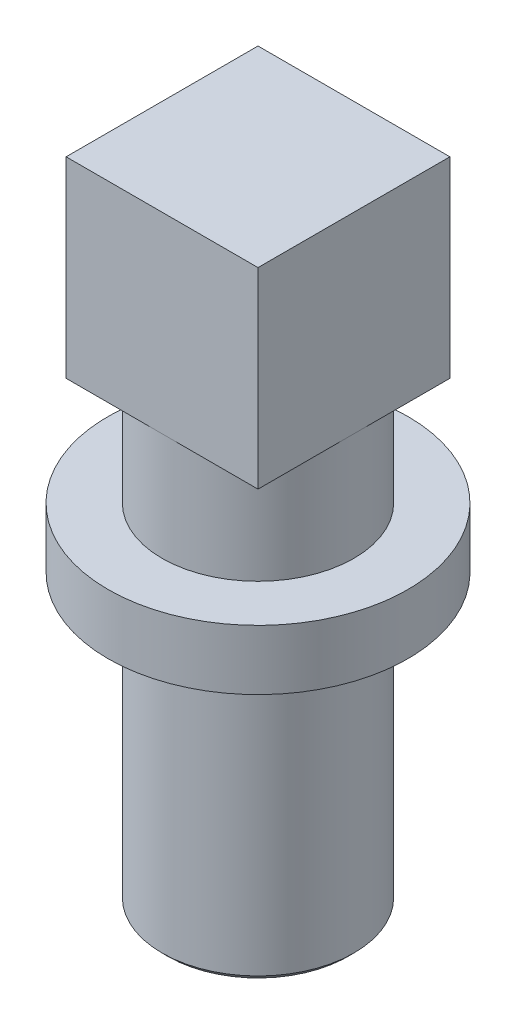
SolidWorks part; units mm, degrees
material "Plain Carbon Steel"
ref_plane "Front Plane" through (0, 0, 0) normal (0, 0, 1) x (1, 0, 0)
ref_plane "Top Plane" through (0, 0, 0) normal (0, 1, 0) x (1, 0, 0)
ref_plane "Right Plane" through (0, 0, 0) normal (1, 0, 0) x (0, 0, -1)
sketch "Shank Sketch Ø16" plane through (0, 0, 0) normal (0, 1, 0) x (1, 0, 0)
  circle A0 centre (0, 0) radius 8
  dimension "D1" = 16
extrude "Shank Ø16x24" add sketch "Shank Sketch Ø16" along normal blind 24
chamfer "Shank End Chamfer 0.5x45" distance 0.5 angle 45 1 edges at (0, 0, 8)
sketch "Collar Sketch Ø25" plane through (0, 24, 0) normal (0, 1, 0) x (1, 0, 0)
  circle A0 centre (0, 0) radius 12.5
  dimension "D1" = 25
extrude "Collar Ø25x5" add sketch "Collar Sketch Ø25" along normal blind 5
sketch "Neck Sketch Ø16" plane through (0, 29, 0) normal (0, 1, 0) x (1, 0, 0)
  circle A0 centre (0, 0) radius 8
  dimension "D1" = 16
extrude "Neck Ø16x9" add sketch "Neck Sketch Ø16" along normal blind 9
sketch "Square Head Sketch 16x16" plane through (0, 38, 0) normal (0, 1, 0) x (1, 0, 0)
  line L1 (-8, -8) -> (8, -8)
  line L2 (-8, -8) -> (-8, 8)
  line L3 (-8, 8) -> (8, 8)
  line L4 (8, -8) -> (8, 8)
  line L5 (-8, -8) -> (8, 8) construction
  line L6 (-8, 8) -> (8, -8) construction
  point P0 (0, 0)
  dimension "D1" = 16
  dimension "D2" = 16
extrude "Square Head 16x16x16" add sketch "Square Head Sketch 16x16" along normal blind 16
